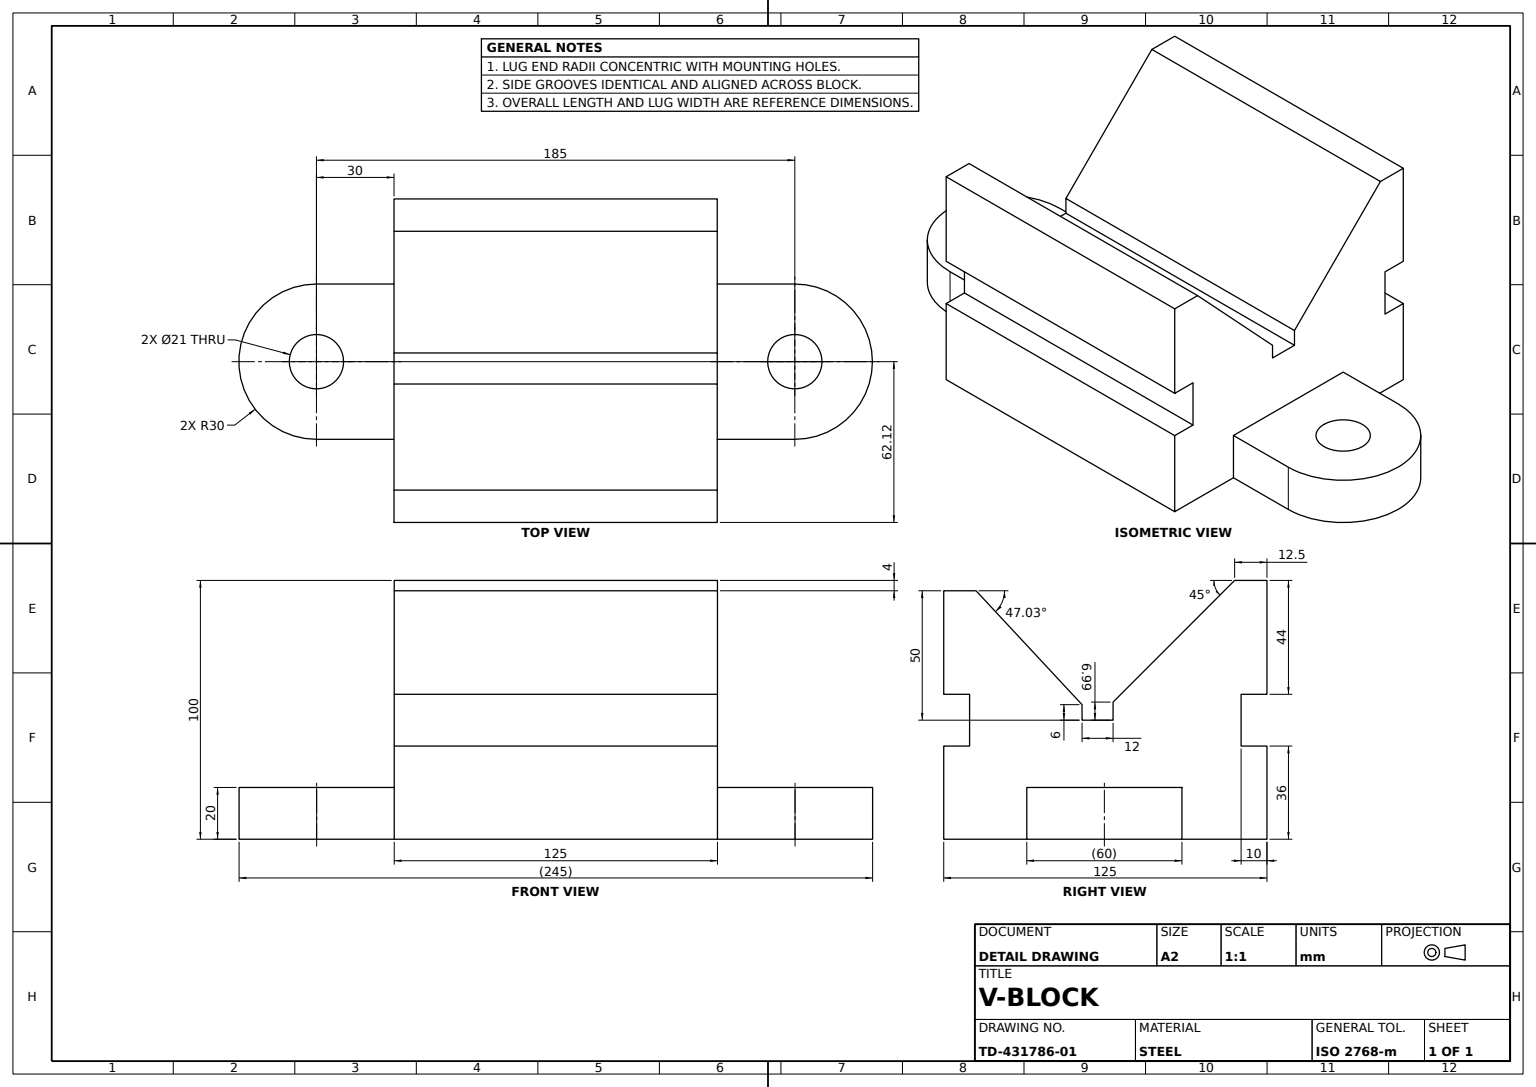
from build123d import *

# Parameters (mm, degrees)
V_BLOCK_BODY_DEPTH     = 125
MOUNTING_LUGS_SKETCH_R = 10.5
MOUNTING_LUGS_DEPTH    = 20


with BuildPart() as part:
    # V-Block Profile Sketch → V-Block Body (new body)
    with BuildSketch(Plane.XY):
        Polygon((-40.458015267, 0), (84.541984733, 0), (84.541984733, 36), (74.541984733, 36), (74.541984733, 56), (84.541984733, 56), (84.541984733, 96), (72.041984733, 96), (31.052534351, 52), (31.052534351, 46), (19.052534351, 46), (19.052534351, 52.989450382), (-27.958015267, 100), (-40.458015267, 100), (-40.458015267, 56), (-30.458015267, 56), (-30.458015267, 36), (-40.458015267, 36), align=None)
    extrude(amount=V_BLOCK_BODY_DEPTH)

    # Mounting Lugs Sketch → Mounting Lugs (add)
    with BuildSketch(Plane.XZ):
        with BuildLine():
            Line((52.421361688, 155), (52.421361688, -30))
            ThreePointArc((52.421361688, -30), (22.421361688, -60), (-7.578638312, -30))
            Line((-7.578638312, -30), (-7.578638312, 155))
            ThreePointArc((-7.578638312, 155), (22.421361688, 185), (52.421361688, 155))
        make_face()
        with Locations(Location((22.421361688, 155, 0), (0, 0, 270))):
            Circle(MOUNTING_LUGS_SKETCH_R, mode=Mode.SUBTRACT)
        with Locations(Location((22.421361688, -30, 0), (0, 0, 270))):
            Circle(MOUNTING_LUGS_SKETCH_R, mode=Mode.SUBTRACT)
    extrude(amount=-MOUNTING_LUGS_DEPTH)


solid = part.part
